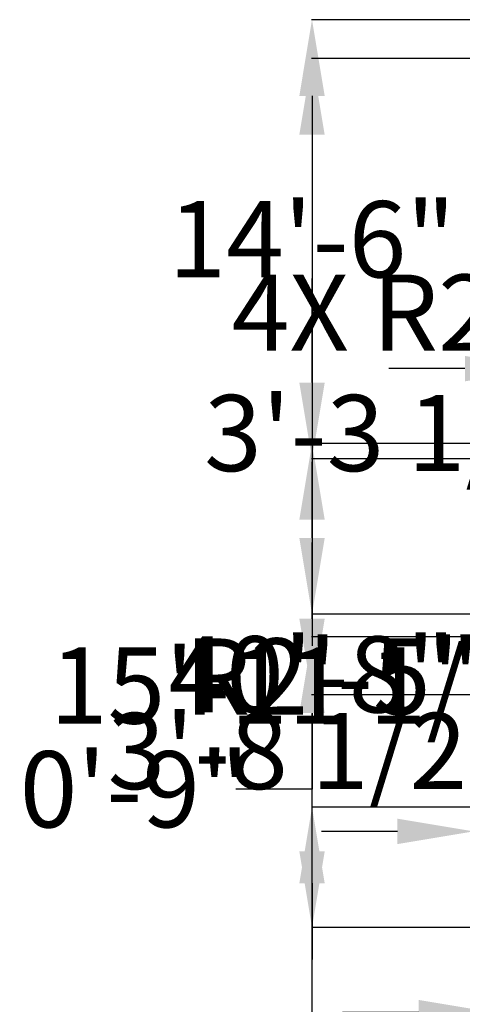
# Model space of a CAD drawing. Units: inches. Extents: x 7323 to 9737, y 2037 to 3322.
# Tile 2 of 19: x 8471 to 8647, y 2297 to 2687. Entities that reach past the tile are written whole.
import ezdxf

# ---------------------------------------------------------------- set-up
doc = ezdxf.new("R2010")
doc.units = ezdxf.units.IN
doc.header["$MEASUREMENT"] = 0
doc.layers.add('A-ANNO-DIMS', color=2, linetype='Continuous', lineweight=18)
doc.styles.get("Standard").update_dxf_attribs({"font": 'arial.ttf'})
doc.dimstyles.get("Standard").update_dxf_attribs({"dimtxt": 30.18, "dimasz": 30.18, "dimexe": 0.18, "dimexo": 0.0625, "dimgap": 0.09, "dimtad": 0, "dimtih": 1, "dimtoh": 1, "dimdec": 0, "dimzin": 0, "dimdsep": 46, "dimlunit": 3, "dimtxsty": 'Standard', "dimcen": 0.09, "dimadec": 0, "dimazin": 0, "dimtfac": 1, "dimtdec": 0, "dimtofl": 0, "dimtmove": 0, "dimatfit": 3, "dimfxl": 1, "dimtolj": 1, "dimtzin": 0, "dimarcsym": 0})

# ---------------------------------------------------------------- blocks, each defined once
blk = doc.blocks.new('*D39')
at = {"layer": 'A-ANNO-DIMS', "color": 0, "lineweight": -2, "transparency": 16777216}
for p, q in [((8647.94, 2549.03), (8617.76, 2549.03)), ((8678.12, 2543.2), (8678.12, 2549.21)), ((8717.39, 2543.2), (8717.39, 2549.21)), ((8747.57, 2549.03), (8777.75, 2549.03))]:
    blk.add_line(p, q, dxfattribs=at)
at = {"layer": 'A-ANNO-DIMS', "color": 0, "transparency": 16777216}
for points in [[(8647.94, 2554.06), (8647.94, 2544), (8678.12, 2549.03)], [(8747.57, 2554.06), (8747.57, 2544), (8717.39, 2549.03)]]:
    blk.add_solid(points, dxfattribs=at)
at = {"layer": 'Defpoints', "color": 0, "transparency": 16777216}
for p in [(8717.39, 2549.03), (8678.12, 2543.14), (8717.39, 2543.14)]:
    blk.add_point(p, dxfattribs=at)
at = {"layer": 'A-ANNO-DIMS', "color": 0, "transparency": 16777216, "insert": (9057.19, 2549.03), "char_height": 30.18, "attachment_point": 5}
blk.add_mtext('\\A1;SINGLE DOOR 3\'-3 1/2" TYP.', dxfattribs=at)
blk = doc.blocks.new('*D40')
at = {"layer": 'A-ANNO-DIMS', "color": 0, "lineweight": -2, "transparency": 16777216}
for p, q in [((8672.23, 2573.32), (8672.23, 2603.5)), ((8678.06, 2543.14), (8672.05, 2543.14)), ((8678.06, 2503.86), (8672.05, 2503.86)), ((8672.23, 2473.68), (8672.23, 2443.5))]:
    blk.add_line(p, q, dxfattribs=at)
at = {"layer": 'A-ANNO-DIMS', "color": 0, "transparency": 16777216}
for points in [[(8667.2, 2573.32), (8677.26, 2573.32), (8672.23, 2543.14)], [(8667.2, 2473.68), (8677.26, 2473.68), (8672.23, 2503.86)]]:
    blk.add_solid(points, dxfattribs=at)
at = {"layer": 'Defpoints', "color": 0, "transparency": 16777216}
for p in [(8672.23, 2543.14), (8678.12, 2543.14), (8678.12, 2503.86)]:
    blk.add_point(p, dxfattribs=at)
at = {"layer": 'A-ANNO-DIMS', "color": 0, "transparency": 16777216, "insert": (8672.23, 2523.5), "char_height": 30.18, "attachment_point": 5}
blk.add_mtext('\\A1;3\'-3 1/2" TYP.', dxfattribs=at)
blk = doc.blocks.new('*D42')
at = {"layer": 'A-ANNO-DIMS', "color": 0, "lineweight": -2, "transparency": 16777216}
for p, q in [((8651.39, 2369.8), (8651.39, 2365.48)), ((8657.39, 2369.8), (8657.39, 2365.48)), ((8621.21, 2365.66), (8591.03, 2365.66)), ((8687.57, 2365.66), (8717.75, 2365.66))]:
    blk.add_line(p, q, dxfattribs=at)
at = {"layer": 'A-ANNO-DIMS', "color": 0, "transparency": 16777216}
for points in [[(8621.21, 2370.69), (8621.21, 2360.63), (8651.39, 2365.66)], [(8687.57, 2370.69), (8687.57, 2360.63), (8657.39, 2365.66)]]:
    blk.add_solid(points, dxfattribs=at)
at = {"layer": 'Defpoints', "color": 0, "transparency": 16777216}
for p in [(8651.39, 2369.86), (8657.39, 2369.86), (8657.39, 2365.66)]:
    blk.add_point(p, dxfattribs=at)
at = {"layer": 'A-ANNO-DIMS', "color": 0, "transparency": 16777216, "insert": (8809.82, 2365.66), "char_height": 30.18, "attachment_point": 5}
blk.add_mtext('\\A1;0\'-6" TYP.', dxfattribs=at)
blk = doc.blocks.new('*D75')
at = {"layer": 'A-ANNO-DIMS', "color": 0, "lineweight": -2, "transparency": 16777216}
for p, q in [((8629.63, 2293.84), (8599.45, 2293.84)), ((8659.81, 2292), (8659.81, 2294.02)), ((8672.52, 2292), (8672.52, 2294.02)), ((8702.7, 2293.84), (8732.88, 2293.84))]:
    blk.add_line(p, q, dxfattribs=at)
at = {"layer": 'A-ANNO-DIMS', "color": 0, "transparency": 16777216}
for points in [[(8629.63, 2298.87), (8629.63, 2288.81), (8659.81, 2293.84)], [(8702.7, 2298.87), (8702.7, 2288.81), (8672.52, 2293.84)]]:
    blk.add_solid(points, dxfattribs=at)
at = {"layer": 'Defpoints', "color": 0, "transparency": 16777216}
for p in [(8659.81, 2291.93), (8672.52, 2293.84), (8672.52, 2291.93)]:
    blk.add_point(p, dxfattribs=at)
at = {"layer": 'A-ANNO-DIMS', "color": 0, "transparency": 16777216, "insert": (9002.27, 2293.84), "char_height": 30.18, "attachment_point": 5}
blk.add_mtext('\\A1;NIGHTSTAND 1\'-0 1/2" TYP.', dxfattribs=at)
blk = doc.blocks.new('*D81')
at = {"layer": 'A-ANNO-DIMS', "color": 0, "lineweight": -2, "transparency": 16777216}
for p, q in [((8651.33, 2671.86), (8587.16, 2671.86)), ((8587.34, 2641.68), (8587.34, 2443.36)), ((8587.34, 2214.04), (8587.34, 2412.36)), ((8651.33, 2183.86), (8587.16, 2183.86))]:
    blk.add_line(p, q, dxfattribs=at)
at = {"layer": 'A-ANNO-DIMS', "color": 0, "transparency": 16777216}
for points in [[(8582.31, 2641.68), (8592.37, 2641.68), (8587.34, 2671.86)], [(8582.31, 2214.04), (8592.37, 2214.04), (8587.34, 2183.86)]]:
    blk.add_solid(points, dxfattribs=at)
at = {"layer": 'Defpoints', "color": 0, "transparency": 16777216}
for p in [(8587.34, 2671.86), (8651.39, 2671.86), (8651.39, 2183.86)]:
    blk.add_point(p, dxfattribs=at)
at = {"layer": 'A-ANNO-DIMS', "color": 0, "transparency": 16777216, "insert": (8587.34, 2427.86), "char_height": 30.18, "attachment_point": 5}
blk.add_mtext('\\A1;40\'-8"', dxfattribs=at)
blk = doc.blocks.new('*D100')
at = {"layer": 'A-ANNO-DIMS', "color": 0, "lineweight": -2, "transparency": 16777216}
for p, q in [((9007.88, 2687.3), (8587.16, 2687.3)), ((8587.34, 2657.12), (8587.34, 2615.8)), ((8587.34, 2543.49), (8587.34, 2584.8)), ((9008.12, 2513.31), (8587.16, 2513.31))]:
    blk.add_line(p, q, dxfattribs=at)
at = {"layer": 'A-ANNO-DIMS', "color": 0, "transparency": 16777216}
for points in [[(8582.31, 2657.12), (8592.37, 2657.12), (8587.34, 2687.3)], [(8582.31, 2543.49), (8592.37, 2543.49), (8587.34, 2513.31)]]:
    blk.add_solid(points, dxfattribs=at)
at = {"layer": 'Defpoints', "color": 0, "transparency": 16777216}
for p in [(9007.95, 2687.3), (8587.34, 2513.31), (9008.18, 2513.31)]:
    blk.add_point(p, dxfattribs=at)
at = {"layer": 'A-ANNO-DIMS', "color": 0, "transparency": 16777216, "insert": (8587.34, 2600.3), "char_height": 30.18, "attachment_point": 5}
blk.add_mtext('\\A1;14\'-6"', dxfattribs=at)
blk = doc.blocks.new('*D106')
at = {"layer": 'A-ANNO-DIMS', "color": 0, "lineweight": -2, "transparency": 16777216}
for p, q in [((9008.12, 2519.31), (8587.16, 2519.31)), ((8587.34, 2489.13), (8587.34, 2439.14)), ((8587.34, 2357.76), (8587.34, 2407.75)), ((9008.23, 2327.58), (8587.16, 2327.58))]:
    blk.add_line(p, q, dxfattribs=at)
at = {"layer": 'A-ANNO-DIMS', "color": 0, "transparency": 16777216}
for points in [[(8582.31, 2489.13), (8592.37, 2489.13), (8587.34, 2519.31)], [(8582.31, 2357.76), (8592.37, 2357.76), (8587.34, 2327.58)]]:
    blk.add_solid(points, dxfattribs=at)
at = {"layer": 'Defpoints', "color": 0, "transparency": 16777216}
for p in [(8587.34, 2519.31), (9008.18, 2519.31), (9008.29, 2327.58)]:
    blk.add_point(p, dxfattribs=at)
at = {"layer": 'A-ANNO-DIMS', "color": 0, "transparency": 16777216, "insert": (8587.34, 2423.44), "char_height": 30.18, "attachment_point": 5}
blk.add_mtext('\\A1;15\'-11 1/2"', dxfattribs=at)
blk = doc.blocks.new('*D108')
at = {"layer": 'A-ANNO-DIMS', "color": 0, "lineweight": -2, "transparency": 16777216}
for p, q in [((8587.34, 2481.93), (8587.34, 2512.11)), ((8841.54, 2451.75), (8587.16, 2451.75)), ((8839.88, 2442.71), (8587.16, 2442.71)), ((8587.34, 2412.53), (8587.34, 2382.35)), ((8587.34, 2382.35), (8557.16, 2382.35))]:
    blk.add_line(p, q, dxfattribs=at)
at = {"layer": 'A-ANNO-DIMS', "color": 0, "transparency": 16777216}
for points in [[(8582.31, 2481.93), (8592.37, 2481.93), (8587.34, 2451.75)], [(8582.31, 2412.53), (8592.37, 2412.53), (8587.34, 2442.71)]]:
    blk.add_solid(points, dxfattribs=at)
at = {"layer": 'Defpoints', "color": 0, "transparency": 16777216}
for p in [(8841.6, 2451.75), (8587.34, 2442.71), (8839.94, 2442.71)]:
    blk.add_point(p, dxfattribs=at)
at = {"layer": 'A-ANNO-DIMS', "color": 0, "transparency": 16777216, "insert": (8516.96, 2382.35), "char_height": 30.18, "attachment_point": 5}
blk.add_mtext('\\A1;0\'-9"', dxfattribs=at)
blk = doc.blocks.new('*D110')
at = {"layer": 'A-ANNO-DIMS', "color": 0, "lineweight": -2, "transparency": 16777216}
for p, q in [((8587.34, 2449.91), (8587.34, 2480.09)), ((9018.85, 2419.73), (8587.16, 2419.73)), ((9018.85, 2375.3), (8587.16, 2375.3)), ((8587.34, 2345.12), (8587.34, 2314.94))]:
    blk.add_line(p, q, dxfattribs=at)
at = {"layer": 'A-ANNO-DIMS', "color": 0, "transparency": 16777216}
for points in [[(8582.31, 2449.91), (8592.37, 2449.91), (8587.34, 2419.73)], [(8582.31, 2345.12), (8592.37, 2345.12), (8587.34, 2375.3)]]:
    blk.add_solid(points, dxfattribs=at)
at = {"layer": 'Defpoints', "color": 0, "transparency": 16777216}
for p in [(8587.34, 2419.73), (9018.91, 2419.73), (9018.91, 2375.3)]:
    blk.add_point(p, dxfattribs=at)
at = {"layer": 'A-ANNO-DIMS', "color": 0, "transparency": 16777216, "insert": (8587.34, 2397.51), "char_height": 30.18, "attachment_point": 5}
blk.add_mtext('\\A1;3\'-8 1/2"', dxfattribs=at)
blk = doc.blocks.new('*D124')
at = {"layer": 'A-ANNO-DIMS', "color": 0, "lineweight": -2, "transparency": 16777216}
for p, q in [((8752.73, 2571.2), (8782.91, 2571.2)), ((8782.91, 2571.2), (8803.63, 2549.26)), ((8848.3, 2501.86), (8848.48, 2501.86)), ((8848.39, 2501.77), (8848.39, 2501.95))]:
    blk.add_line(p, q, dxfattribs=at)
at = {"layer": 'A-ANNO-DIMS', "color": 0, "transparency": 16777216}
blk.add_solid([(8807.29, 2552.71), (8799.97, 2545.81), (8824.35, 2527.32)], dxfattribs=at)
at = {"layer": 'Defpoints', "color": 0, "transparency": 16777216}
for p in [(8824.35, 2527.32), (8848.39, 2501.86)]:
    blk.add_point(p, dxfattribs=at)
at = {"layer": 'A-ANNO-DIMS', "color": 0, "transparency": 16777216, "insert": (8653.33, 2571.2), "char_height": 30.18, "attachment_point": 5}
blk.add_mtext('\\A1;4X R2\'-11"', dxfattribs=at)
blk = doc.blocks.new('*D125')
at = {"layer": 'A-ANNO-DIMS', "color": 0, "lineweight": -2, "transparency": 16777216}
for p, q in [((8650, 2427.05), (8680.18, 2427.05)), ((8680.18, 2427.05), (8701.53, 2405.72)), ((8743.3, 2363.86), (8743.48, 2363.86)), ((8743.39, 2363.77), (8743.39, 2363.95))]:
    blk.add_line(p, q, dxfattribs=at)
at = {"layer": 'A-ANNO-DIMS', "color": 0, "transparency": 16777216}
blk.add_solid([(8705.08, 2409.27), (8697.97, 2402.16), (8722.87, 2384.38)], dxfattribs=at)
at = {"layer": 'Defpoints', "color": 0, "transparency": 16777216}
for p in [(8722.87, 2384.38), (8743.39, 2363.86)]:
    blk.add_point(p, dxfattribs=at)
at = {"layer": 'A-ANNO-DIMS', "color": 0, "transparency": 16777216, "insert": (8595.36, 2427.05), "char_height": 30.18, "attachment_point": 5}
blk.add_mtext('\\A1;R2\'-5"', dxfattribs=at)

msp = doc.modelspace()

# ---------------------------------------------------------------- dimensions: what is measured, and where the dimension line sits
at = {"layer": 'A-ANNO-DIMS'}
for base, p1, p2, picture, middle in [((8587.34, 2513.31), (9007.95, 2687.3), (9008.18, 2513.31), '*D100', (8587.34, 2600.3)), ((8587.34, 2671.86), (8651.39, 2183.86), (8651.39, 2671.86), '*D81', (8587.34, 2427.86)), ((8587.34, 2519.31), (9008.29, 2327.58), (9008.18, 2519.31), '*D106', (8587.34, 2423.44)), ((8587.34, 2442.71), (8841.6, 2451.75), (8839.94, 2442.71), '*D108', (8516.96, 2382.35)), ((8587.34, 2419.73), (9018.91, 2375.3), (9018.91, 2419.73), '*D110', (8587.34, 2397.51))]:
    dim = msp.add_linear_dim(base=base, p1=p1, p2=p2, angle=90, dimstyle='Standard', override={"dimdec": 1, "dimlfac": 1, "dimrnd": 0, "dimzin": 1, "dimdsep": 46, "dimlunit": 4, "dimfrac": 2}, dxfattribs=at)
    dim.commit()
    dim.dimension.update_dxf_attribs({"geometry": picture, "text_midpoint": middle})
for base, p1, p2, text, picture, middle in [((8717.39, 2549.03), (8678.12, 2543.14), (8717.39, 2543.14), 'SINGLE DOOR <> TYP.', '*D39', (9057.19, 2549.03)), ((8657.39, 2365.66), (8651.39, 2369.86), (8657.39, 2369.86), '<> TYP.', '*D42', (8809.82, 2365.66)), ((8672.52, 2293.84), (8659.81, 2291.93), (8672.52, 2291.93), 'NIGHTSTAND <> TYP.', '*D75', (9002.27, 2293.84))]:
    dim = msp.add_linear_dim(base=base, p1=p1, p2=p2, text=text, dimstyle='Standard', override={"dimdec": 1, "dimlfac": 1, "dimrnd": 0, "dimzin": 1, "dimdsep": 46, "dimlunit": 4, "dimfrac": 2}, dxfattribs=at)
    dim.commit()
    dim.dimension.update_dxf_attribs({"geometry": picture, "text_midpoint": middle})
dim = msp.add_radius_dim(center=(8848.39, 2501.86), mpoint=(8824.35, 2527.32), text='4X <>', dimstyle='Standard', override={"dimdec": 1, "dimlfac": 1, "dimrnd": 0, "dimzin": 1, "dimdsep": 46, "dimlunit": 4, "dimfrac": 2}, dxfattribs=at)
dim.commit()
dim.dimension.update_dxf_attribs({"geometry": '*D124', "text_midpoint": (8653.33, 2571.2)})
dim = msp.add_linear_dim(base=(8672.23, 2543.14), p1=(8678.12, 2503.86), p2=(8678.12, 2543.14), angle=90, text='<> TYP.', dimstyle='Standard', override={"dimdec": 1, "dimlfac": 1, "dimrnd": 0, "dimzin": 1, "dimdsep": 46, "dimlunit": 4, "dimfrac": 2}, dxfattribs=at)
dim.commit()
dim.dimension.update_dxf_attribs({"geometry": '*D40', "text_midpoint": (8672.23, 2523.5)})
dim = msp.add_radius_dim(center=(8743.39, 2363.86), mpoint=(8722.87, 2384.38), dimstyle='Standard', override={"dimdec": 1, "dimlfac": 1, "dimrnd": 0, "dimzin": 1, "dimdsep": 46, "dimlunit": 4, "dimfrac": 2}, dxfattribs=at)
dim.commit()
dim.dimension.update_dxf_attribs({"geometry": '*D125', "text_midpoint": (8595.36, 2427.05)})

doc.saveas('drawing.dxf')
